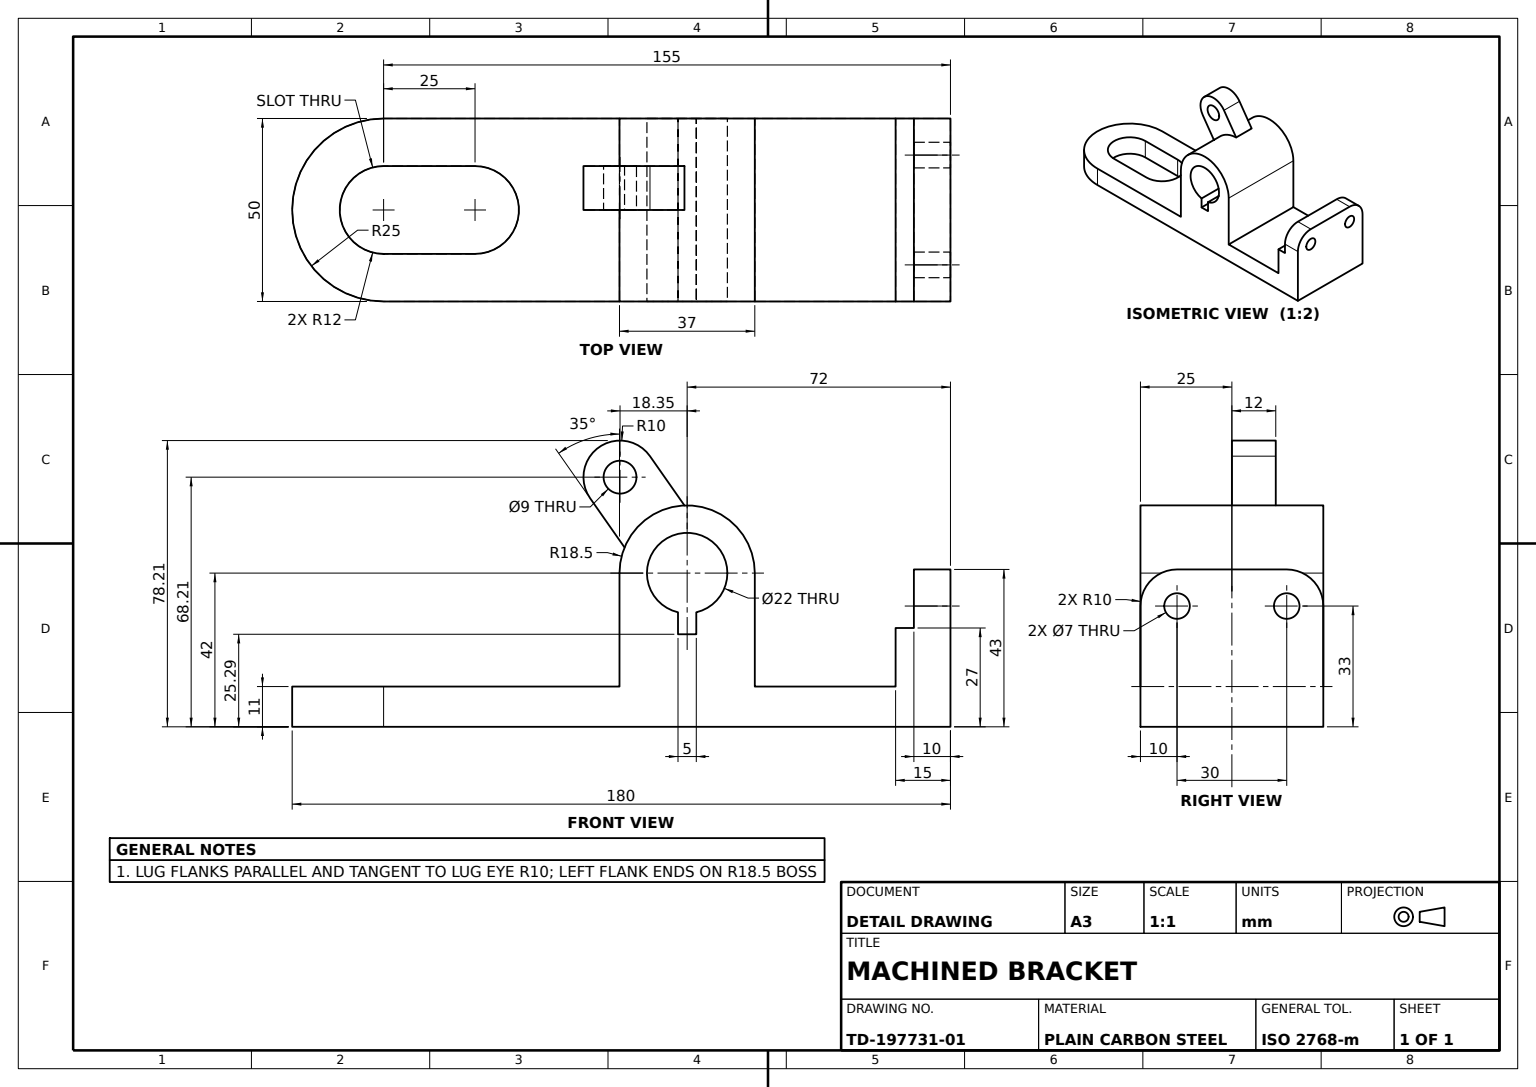
SolidWorks part; units mm, degrees
material "Plain Carbon Steel"
ref_plane "Front Plane" through (0, 0, 0) normal (0, 0, 1) x (1, 0, 0)
ref_plane "Top Plane" through (0, 0, 0) normal (0, 1, 0) x (1, 0, 0)
ref_plane "Right Plane" through (0, 0, 0) normal (1, 0, 0) x (0, 0, -1)
sketch "Base Plate Sketch" plane through (0, 0, 0) normal (0, 1, 0) x (1, 0, 0)
  line L0 (0, 0) -> (-25, 0) construction
  line L1 (0, -12) -> (-25, -12)
  line L2 (0, 12) -> (-25, 12)
  line L3 (0, 25) -> (-155, 25)
  line L4 (0, -25) -> (-155, -25)
  line L5 (-155, -25) -> (-155, 25)
  arc A0 (0, -25) -> (0, 25) centre (0, 0) ccw
  arc A1 (0, -12) -> (0, 12) centre (0, 0) ccw
  arc A2 (-25, 12) -> (-25, -12) centre (-25, 0) ccw
  point P3 (-12.5, 0)
  dimension "D1" = 50
  dimension "D2" = 13
  dimension "D3" = 25
  dimension "D4" = 155
extrude "Slotted Base Plate" add sketch "Base Plate Sketch" along normal blind 11
sketch "Upright Profile Sketch" plane through (0, 0, 25) normal (0, 0, 1) x (1, 0, 0)
  line L0 (-155, 0) -> (-155, 43)
  line L1 (-155, 43) -> (-145, 43)
  line L2 (-145, 43) -> (-145, 27)
  line L3 (-145, 27) -> (-140, 27)
  line L4 (-140, 27) -> (-140, 11)
  line L5 (-155, 11) -> (0, 11) construction
  line L6 (-140, 11) -> (-155, 0)
  line L7 (-155, 0) -> (0, 0) construction
  line L8 (-101.5, 42) -> (-101.5, 11)
  line L9 (-64.5, 42) -> (-64.5, 11)
  line L10 (-101.5, 11) -> (-64.5, 11)
  line L11 (-83, 42) -> (-83, 11)
  line L13 (-85.5, 25.2879) -> (-80.5, 25.2879)
  line L14 (-85.5, 25.2879) -> (-85.5, 31.2879)
  line L16 (-80.5, 25.2879) -> (-80.5, 31.2879)
  arc A0 (-80.5, 31.2879) -> (-85.5, 31.2879) centre (-83, 42) ccw
  arc A1 (-64.5, 42) -> (-101.5, 42) centre (-83, 42) ccw
  point P5 (-150, 43)
  point P12 (-83, 28.7392)
  dimension "D6" = 37
  dimension "D7" = 22
  dimension "D1" = 43
  dimension "D2" = 16
  dimension "D3" = 15
  dimension "D4" = 5
  dimension "D5" = 42
  dimension "D8" = 72
  dimension "D9" = 5
  dimension "D10" = 2.5
  dimension "D11" = 6
  dimension "D12" = 31
  dimension "D13" = 13.2608
extrude "Upright Hub Body" add sketch "Upright Profile Sketch" against normal blind 50
ref_plane "Plane1" through (0, 0, 0) normal (0, 0, 1) x (1, 0, 0)
sketch "Cross Boss Sketch" plane through (0, 0, 0) normal (0, 0, 1) x (1, 0, 0)
  line L3 (-65.8811, 49.0138) -> (-56.454, 62.4771)
  line L6 (-82.2642, 60.4854) -> (-72.8371, 73.9486)
  circle A0 centre (-64.6456, 68.2129) radius 4.5
  arc A1 (-56.454, 62.4771) -> (-72.8371, 73.9486) centre (-64.6456, 68.2129) ccw
  arc A3 (-65.8811, 49.0138) -> (-82.2642, 60.4854) centre (-83, 42) ccw
  dimension "D2" = 20
  dimension "D3" = 9
  dimension "D1" = 18.5
  dimension "D4" = 32
  dimension "D5" = 0.7358
  dimension "D6" = 10.1629
extrude "Cross Boss" add sketch "Cross Boss Sketch" along normal blind 12
fillet "Upright Fillet R10" radius 10 2 edges at (-150, 43, -25) (-150, 43, 25)
sketch "Cross Hole Sketch" plane through (-155, 0, 0) normal (-1, 0, 0) x (0, 0, 1)
  circle A0 centre (15, 33) radius 3.5
  circle A1 centre (-15, 33) radius 3.5
  dimension "D1" = 7
  dimension "D2" = 7
extrude "Cross Hole Cut" cut sketch "Cross Hole Sketch" against normal blind 12
